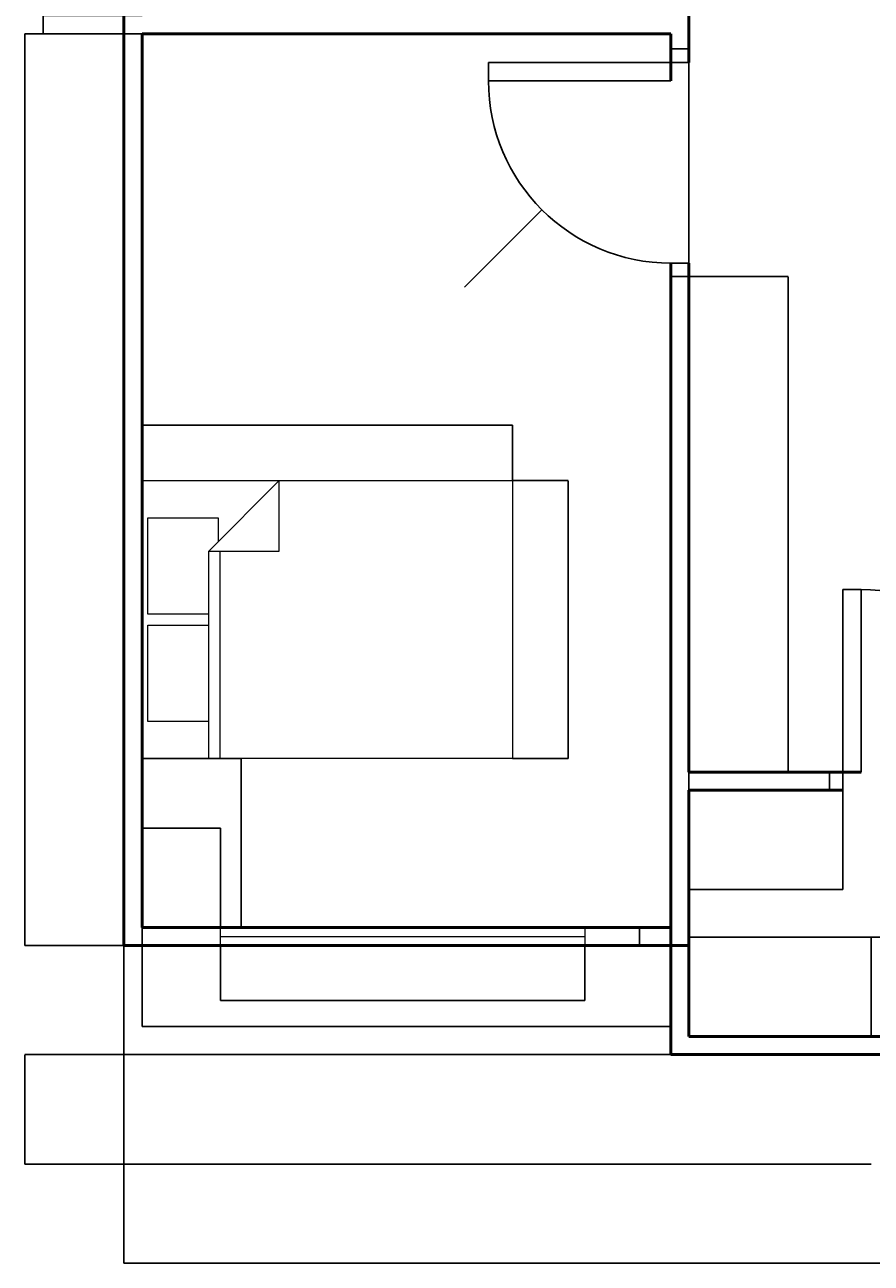
# Model space of a CAD drawing. Units: millimetres. Extents: x 1584 to 12772, y -932 to 10602.
# Tile 1 of 4: x 1584 to 6228, y -932 to 5860. Entities that reach past the tile are written whole.
import ezdxf

# ---------------------------------------------------------------- set-up
doc = ezdxf.new("R2010")
doc.units = ezdxf.units.MM
for name, color, linetype, lineweight in [('A-ANNO-DIMS', 2, 'Continuous', 18), ('A-DOOR', 3, 'Continuous', 25), ('A-FURN', 8, 'Continuous', 18), ('A-GLAZ', 4, 'Continuous', 18), ('A-WALL', 7, 'Continuous', 50)]:
    doc.layers.add(name, color=color, linetype=linetype, lineweight=lineweight)
doc.styles.get("Standard").update_dxf_attribs({"font": 'arial.ttf'})
doc.dimstyles.get("Standard").update_dxf_attribs({"dimtxt": 0.18, "dimasz": 0.18, "dimexe": 0.18, "dimexo": 0.0625, "dimgap": 0.09, "dimtad": 0, "dimtih": 1, "dimtoh": 1, "dimdec": 4, "dimzin": 0, "dimdsep": 46, "dimtxsty": 'Standard', "dimcen": 0.09, "dimadec": 0, "dimazin": 0, "dimtfac": 1, "dimtdec": 4, "dimtofl": 0, "dimtmove": 0, "dimatfit": 3, "dimfxl": 1, "dimtolj": 1, "dimtzin": 0, "dimarcsym": 0})

# ---------------------------------------------------------------- blocks, each defined once
blk = doc.blocks.new('Bed - Queen')
for p, q in [((0, -80.00003), (0, 0)), ((0, 0), (59.99999, 0)), ((59.99999, 0), (59.99999, -80.00003)), ((7.99999, -1.2), (28.79998, -1.2)), ((7.99999, -14.4), (7.99999, -1.2)), ((28.79998, -1.2), (28.79998, -14.4)), ((31.19999, -1.2), (51.99999, -1.2)), ((31.19999, -14.4), (31.19999, -1.2)), ((51.99999, -1.2), (51.99999, -16.4)), ((0, -14.4), (44.8, -14.4)), ((59.99999, -29.6), (44.8, -14.4)), ((44.8, -14.4), (44.8, -29.6)), ((44.8, -16.8), (0, -16.8)), ((51.99999, -16.4), (46.79936, -16.4)), ((44.8, -29.6), (59.99999, -29.6)), ((59.99999, -80.00003), (0, -80.00003))]:
    blk.add_line(p, q)
blk = doc.blocks.new('DOOR-SINGLE-1000')
for p, q in [((1000, 1174.2), (1000, 1248.4)), ((1000, 1248.4), (1100, 1248.4)), ((1100, 1248.4), (1100, 1174.2)), ((1000, 1174.2), (0, 1174.2)), ((0, 1174.2), (0, 1074.2)), ((1000, 1074.2), (1000, 1174.2)), ((1100, 1174.2), (1000, 1174.2)), ((0, 1074.2), (1000, 1074.2)), ((1000, 0), (1000, 74.2)), ((1000, 74.2), (1100, 74.2)), ((1100, 74.2), (1100, 0)), ((1100, 0), (1000, 0))]:
    blk.add_line(p, q)
blk.add_arc((1000, 1074.2), 1000, 180, 270)
blk = doc.blocks.new('DOOR-ENTRY-LEAF-1000')
for p, q in [((1100, 1100), (1000, 1100)), ((1000, 1100), (1000, 100)), ((1100, 100), (1100, 1100)), ((1000, 100), (1100, 100)), ((1100, 100), (1174.2, 100)), ((1100, 0), (1100, 100)), ((1174.2, 100), (1174.2, 0)), ((1174.2, 0), (1100, 0))]:
    blk.add_line(p, q)
blk.add_arc((1000, 100), 1000, 90, 180)
blk = doc.blocks.new('WIN-2000')
for p, q in [((0, 100), (2000, 100)), ((0, 0), (0, 100)), ((2000, 100), (2000, 0)), ((0, 50), (2000, 50)), ((2000, 0), (0, 0))]:
    blk.add_line(p, q)
blk = doc.blocks.new('*D14')
at = {"layer": 'A-ANNO-DIMS', "color": 0, "lineweight": -2, "transparency": 16777216}
for p, q in [((2657.2, 810.1), (2657.2, 510)), ((4657.2, 810.1), (4657.2, 510)), ((2657.4, 510.2), (3656, 510.2)), ((4657, 510.2), (3658.5, 510.2))]:
    blk.add_line(p, q, dxfattribs=at)
at = {"layer": 'A-ANNO-DIMS', "color": 0, "transparency": 16777216}
for points in [[(2657.4, 510.2), (2657.4, 510.2), (2657.2, 510.2)], [(4657, 510.2), (4657, 510.2), (4657.2, 510.2)]]:
    blk.add_solid(points, dxfattribs=at)
at = {"layer": 'Defpoints', "color": 0, "transparency": 16777216}
for p in [(2657.2, 810.2), (4657.2, 810.2), (4657.2, 510.2)]:
    blk.add_point(p, dxfattribs=at)
at = {"layer": 'A-ANNO-DIMS', "color": 0, "transparency": 16777216, "insert": (3657.2, 510.2), "char_height": 0.18, "attachment_point": 5}
blk.add_mtext('\\A1;WINDOW 2000 TYP.', dxfattribs=at)
blk = doc.blocks.new('*D15')
at = {"layer": 'A-ANNO-DIMS', "color": 0, "lineweight": -2, "transparency": 16777216}
for p, q in [((4657.3, 910.2), (4957.4, 910.2)), ((4957.2, 910), (4957.2, 860.4)), ((4957.2, 810.4), (4957.2, 860)), ((4657.3, 810.2), (4957.4, 810.2))]:
    blk.add_line(p, q, dxfattribs=at)
at = {"layer": 'A-ANNO-DIMS', "color": 0, "transparency": 16777216}
for points in [[(4957.2, 910), (4957.3, 910), (4957.2, 910.2)], [(4957.2, 810.4), (4957.3, 810.4), (4957.2, 810.2)]]:
    blk.add_solid(points, dxfattribs=at)
at = {"layer": 'Defpoints', "color": 0, "transparency": 16777216}
for p in [(4657.2, 910.2), (4957.2, 910.2), (4657.2, 810.2)]:
    blk.add_point(p, dxfattribs=at)
at = {"layer": 'A-ANNO-DIMS', "color": 0, "transparency": 16777216, "insert": (4957.2, 860.2), "char_height": 0.18, "attachment_point": 5}
blk.add_mtext('\\A1;100 TYP.', dxfattribs=at)
blk = doc.blocks.new('*D20')
at = {"layer": 'A-ANNO-DIMS', "color": 0, "lineweight": -2, "transparency": 16777216}
for p, q in [((2227.8, 3360.2), (2227.8, 3665.2)), ((2228, 3665), (3242.4, 3665)), ((4259.7, 3665), (3245.3, 3665)), ((4259.8, 3360.2), (4259.8, 3665.2))]:
    blk.add_line(p, q, dxfattribs=at)
at = {"layer": 'A-ANNO-DIMS', "color": 0, "transparency": 16777216}
for points in [[(2228, 3665), (2228, 3665), (2227.8, 3665)], [(4259.7, 3665), (4259.7, 3665), (4259.8, 3665)]]:
    blk.add_solid(points, dxfattribs=at)
at = {"layer": 'Defpoints', "color": 0, "transparency": 16777216}
for p in [(2227.8, 3665), (2227.8, 3360.2), (4259.8, 3360.2)]:
    blk.add_point(p, dxfattribs=at)
at = {"layer": 'A-ANNO-DIMS', "color": 0, "transparency": 16777216, "insert": (3243.8, 3665), "char_height": 0.18, "attachment_point": 5}
blk.add_mtext('\\A1;QUEEN BED 2032 TYP.', dxfattribs=at)
blk = doc.blocks.new('*D21')
at = {"layer": 'A-ANNO-DIMS', "color": 0, "lineweight": -2, "transparency": 16777216}
for p, q in [((4259.9, 3360.2), (4564.8, 3360.2)), ((4564.6, 3360), (4564.6, 2598.4)), ((4564.6, 1836.4), (4564.6, 2598)), ((4259.9, 1836.2), (4564.8, 1836.2))]:
    blk.add_line(p, q, dxfattribs=at)
at = {"layer": 'A-ANNO-DIMS', "color": 0, "transparency": 16777216}
for points in [[(4564.6, 3360), (4564.7, 3360), (4564.6, 3360.2)], [(4564.6, 1836.4), (4564.7, 1836.4), (4564.6, 1836.2)]]:
    blk.add_solid(points, dxfattribs=at)
at = {"layer": 'Defpoints', "color": 0, "transparency": 16777216}
for p in [(4259.8, 3360.2), (4564.6, 3360.2), (4259.8, 1836.2)]:
    blk.add_point(p, dxfattribs=at)
at = {"layer": 'A-ANNO-DIMS', "color": 0, "transparency": 16777216, "insert": (4564.6, 2598.2), "char_height": 0.18, "attachment_point": 5}
blk.add_mtext('\\A1;1524 TYP.', dxfattribs=at)
blk = doc.blocks.new('*D36')
at = {"layer": 'A-ANNO-DIMS', "color": 0, "lineweight": -2, "transparency": 16777216}
for p, q in [((2127.8, 810.1), (2127.8, -931.5)), ((12227.8, 810.1), (12227.8, -931.5)), ((2128, -931.3), (7177.4, -931.3)), ((12227.7, -931.3), (7178.3, -931.3))]:
    blk.add_line(p, q, dxfattribs=at)
at = {"layer": 'A-ANNO-DIMS', "color": 0, "transparency": 16777216}
for points in [[(2128, -931.3), (2128, -931.4), (2127.8, -931.3)], [(12227.7, -931.3), (12227.7, -931.4), (12227.8, -931.3)]]:
    blk.add_solid(points, dxfattribs=at)
at = {"layer": 'Defpoints', "color": 0, "transparency": 16777216}
for p in [(2127.8, 810.2), (12227.8, 810.2), (12227.8, -931.3)]:
    blk.add_point(p, dxfattribs=at)
at = {"layer": 'A-ANNO-DIMS', "color": 0, "transparency": 16777216, "insert": (7177.8, -931.3), "char_height": 0.18, "attachment_point": 5}
blk.add_mtext('\\A1;10100', dxfattribs=at)
blk = doc.blocks.new('*D38')
at = {"layer": 'A-ANNO-DIMS', "color": 0, "lineweight": -2, "transparency": 16777216}
for p, q in [((2227.8, 5810.2), (1584, 5810.2)), ((1584.1, 5810), (1584.1, 3310.4)), ((1584.1, 810.4), (1584.1, 3310)), ((2127.8, 810.2), (1584, 810.2))]:
    blk.add_line(p, q, dxfattribs=at)
at = {"layer": 'A-ANNO-DIMS', "color": 0, "transparency": 16777216}
for points in [[(1584.1, 5810), (1584.2, 5810), (1584.1, 5810.2)], [(1584.1, 810.4), (1584.2, 810.4), (1584.1, 810.2)]]:
    blk.add_solid(points, dxfattribs=at)
at = {"layer": 'Defpoints', "color": 0, "transparency": 16777216}
for p in [(1584.1, 5810.2), (2227.8, 5810.2), (2127.8, 810.2)]:
    blk.add_point(p, dxfattribs=at)
at = {"layer": 'A-ANNO-DIMS', "color": 0, "transparency": 16777216, "insert": (1584.1, 3310.2), "char_height": 0.18, "attachment_point": 5}
blk.add_mtext('\\A1;5000', dxfattribs=at)
blk = doc.blocks.new('*D40')
at = {"layer": 'A-ANNO-DIMS', "color": 0, "lineweight": -2, "transparency": 16777216}
for p, q in [((2227.8, 5910.2), (1684, 5910.2)), ((1684.1, 5910), (1684.1, 5860.4)), ((1684.1, 5810.4), (1684.1, 5860)), ((2227.8, 5810.2), (1684, 5810.2))]:
    blk.add_line(p, q, dxfattribs=at)
at = {"layer": 'A-ANNO-DIMS', "color": 0, "transparency": 16777216}
for points in [[(1684.1, 5910), (1684.2, 5910), (1684.1, 5910.2)], [(1684.1, 5810.4), (1684.2, 5810.4), (1684.1, 5810.2)]]:
    blk.add_solid(points, dxfattribs=at)
at = {"layer": 'Defpoints', "color": 0, "transparency": 16777216}
for p in [(1684.1, 5910.2), (2227.8, 5910.2), (2227.8, 5810.2)]:
    blk.add_point(p, dxfattribs=at)
at = {"layer": 'A-ANNO-DIMS', "color": 0, "transparency": 16777216, "insert": (1684.1, 5860.2), "char_height": 0.18, "attachment_point": 5}
blk.add_mtext('\\A1;100', dxfattribs=at)
blk = doc.blocks.new('*D43')
at = {"layer": 'A-ANNO-DIMS', "color": 0, "lineweight": -2, "transparency": 16777216}
for p, q in [((2227.83323, 910.118106), (2227.83323, 366.300606)), ((5127.83323, 910.118106), (5127.83323, 366.300606)), ((2228.01323, 366.480606), (3677.47323, 366.480606)), ((5127.65323, 366.480606), (3678.19323, 366.480606))]:
    blk.add_line(p, q, dxfattribs=at)
at = {"layer": 'A-ANNO-DIMS', "color": 0, "transparency": 16777216}
for points in [[(2228.01323, 366.510606), (2228.01323, 366.450606), (2227.83323, 366.480606)], [(5127.65323, 366.510606), (5127.65323, 366.450606), (5127.83323, 366.480606)]]:
    blk.add_solid(points, dxfattribs=at)
at = {"layer": 'Defpoints', "color": 0, "transparency": 16777216}
for p in [(2227.83323, 910.180606), (5127.83323, 910.180606), (2227.83323, 366.480606)]:
    blk.add_point(p, dxfattribs=at)
at = {"layer": 'A-ANNO-DIMS', "color": 0, "transparency": 16777216, "insert": (3677.83323, 366.480606), "char_height": 0.18, "attachment_point": 5}
blk.add_mtext('\\A1;2900', dxfattribs=at)
blk = doc.blocks.new('*D44')
at = {"layer": 'A-ANNO-DIMS', "color": 0, "lineweight": -2, "transparency": 16777216}
for p, q in [((5227.8, 312.4), (5227.8, 10454.1)), ((5228, 10453.9), (7177.5, 10453.9)), ((9127.7, 10453.9), (7178.2, 10453.9)), ((9127.8, 312.4), (9127.8, 10454.1))]:
    blk.add_line(p, q, dxfattribs=at)
at = {"layer": 'A-ANNO-DIMS', "color": 0, "transparency": 16777216}
for points in [[(5228, 10453.9), (5228, 10453.9), (5227.8, 10453.9)], [(9127.7, 10453.9), (9127.7, 10453.9), (9127.8, 10453.9)]]:
    blk.add_solid(points, dxfattribs=at)
at = {"layer": 'Defpoints', "color": 0, "transparency": 16777216}
for p in [(9127.8, 10453.9), (5227.8, 312.4), (9127.8, 312.4)]:
    blk.add_point(p, dxfattribs=at)
at = {"layer": 'A-ANNO-DIMS', "color": 0, "transparency": 16777216, "insert": (7177.8, 10453.9), "char_height": 0.18, "attachment_point": 5}
blk.add_mtext('\\A1;3900', dxfattribs=at)
blk = doc.blocks.new('*D47')
at = {"layer": 'A-ANNO-DIMS', "color": 0, "lineweight": -2, "transparency": 16777216}
for p, q in [((6227.83323, 312.424388), (6227.83323, 856.241888)), ((6228.01323, 856.061888), (7227.47323, 856.061888)), ((8227.65323, 856.061888), (7228.19323, 856.061888)), ((8227.83323, 312.424388), (8227.83323, 856.241888))]:
    blk.add_line(p, q, dxfattribs=at)
at = {"layer": 'A-ANNO-DIMS', "color": 0, "transparency": 16777216}
for points in [[(6228.01323, 856.091888), (6228.01323, 856.031888), (6227.83323, 856.061888)], [(8227.65323, 856.091888), (8227.65323, 856.031888), (8227.83323, 856.061888)]]:
    blk.add_solid(points, dxfattribs=at)
at = {"layer": 'Defpoints', "color": 0, "transparency": 16777216}
for p in [(8227.83323, 856.061888), (6227.83323, 312.361888), (8227.83323, 312.361888)]:
    blk.add_point(p, dxfattribs=at)
at = {"layer": 'A-ANNO-DIMS', "color": 0, "transparency": 16777216, "insert": (7227.83323, 856.061888), "char_height": 0.18, "attachment_point": 5}
blk.add_mtext('\\A1;2000', dxfattribs=at)
blk = doc.blocks.new('*D48')
at = {"layer": 'A-ANNO-DIMS', "color": 0, "lineweight": -2, "transparency": 16777216}
for p, q in [((5227.8, 312.4), (5227.8, 856.2)), ((5228, 856.1), (5727.5, 856.1)), ((6227.7, 856.1), (5728.2, 856.1)), ((6227.8, 312.4), (6227.8, 856.2))]:
    blk.add_line(p, q, dxfattribs=at)
at = {"layer": 'A-ANNO-DIMS', "color": 0, "transparency": 16777216}
for points in [[(5228, 856.1), (5228, 856), (5227.8, 856.1)], [(6227.7, 856.1), (6227.7, 856), (6227.8, 856.1)]]:
    blk.add_solid(points, dxfattribs=at)
at = {"layer": 'Defpoints', "color": 0, "transparency": 16777216}
for p in [(6227.8, 856.1), (5227.8, 312.4), (6227.8, 312.4)]:
    blk.add_point(p, dxfattribs=at)
at = {"layer": 'A-ANNO-DIMS', "color": 0, "transparency": 16777216, "insert": (5727.8, 856.1), "char_height": 0.18, "attachment_point": 5}
blk.add_mtext('\\A1;1000', dxfattribs=at)
blk = doc.blocks.new('*D49')
at = {"layer": 'A-ANNO-DIMS', "color": 0, "lineweight": -2, "transparency": 16777216}
for p, q in [((5127.8, 212.4), (1584, 212.4)), ((1584.1, 212.2), (1584.1, -87.5)), ((1584.1, -387.5), (1584.1, -87.8)), ((6227.8, -387.6), (1584, -387.6))]:
    blk.add_line(p, q, dxfattribs=at)
at = {"layer": 'A-ANNO-DIMS', "color": 0, "transparency": 16777216}
for points in [[(1584.1, 212.2), (1584.2, 212.2), (1584.1, 212.4)], [(1584.1, -387.5), (1584.2, -387.5), (1584.1, -387.6)]]:
    blk.add_solid(points, dxfattribs=at)
at = {"layer": 'Defpoints', "color": 0, "transparency": 16777216}
for p in [(5127.8, 212.4), (1584.1, -387.6), (6227.8, -387.6)]:
    blk.add_point(p, dxfattribs=at)
at = {"layer": 'A-ANNO-DIMS', "color": 0, "transparency": 16777216, "insert": (1584.1, -87.6), "char_height": 0.18, "attachment_point": 5}
blk.add_mtext('\\A1;600', dxfattribs=at)
blk = doc.blocks.new('*D50')
at = {"layer": 'A-ANNO-DIMS', "color": 0, "lineweight": -2, "transparency": 16777216}
for p, q in [((5227.8, 1662.3), (5227.8, 1118.5)), ((6072.8, 1662.3), (6072.8, 1118.5)), ((5228, 1118.7), (5650, 1118.7)), ((6072.6, 1118.7), (5650.6, 1118.7))]:
    blk.add_line(p, q, dxfattribs=at)
at = {"layer": 'A-ANNO-DIMS', "color": 0, "transparency": 16777216}
for points in [[(5228, 1118.7), (5228, 1118.6), (5227.8, 1118.7)], [(6072.6, 1118.7), (6072.6, 1118.6), (6072.8, 1118.7)]]:
    blk.add_solid(points, dxfattribs=at)
at = {"layer": 'Defpoints', "color": 0, "transparency": 16777216}
for p in [(5227.8, 1662.4), (6072.8, 1662.4), (5227.8, 1118.7)]:
    blk.add_point(p, dxfattribs=at)
at = {"layer": 'A-ANNO-DIMS', "color": 0, "transparency": 16777216, "insert": (5650.3, 1118.7), "char_height": 0.18, "attachment_point": 5}
blk.add_mtext('\\A1;845', dxfattribs=at)
blk = doc.blocks.new('*D54')
at = {"layer": 'A-ANNO-DIMS', "color": 0, "lineweight": -2, "transparency": 16777216}
for p, q in [((2227.8, 910.2), (2227.8, 1454.1)), ((2228, 1453.9), (2442.1, 1453.9)), ((2657, 1453.9), (2442.9, 1453.9)), ((2657.2, 910.2), (2657.2, 1454.1))]:
    blk.add_line(p, q, dxfattribs=at)
at = {"layer": 'A-ANNO-DIMS', "color": 0, "transparency": 16777216}
for points in [[(2228, 1453.9), (2228, 1453.9), (2227.8, 1453.9)], [(2657, 1453.9), (2657, 1453.9), (2657.2, 1453.9)]]:
    blk.add_solid(points, dxfattribs=at)
at = {"layer": 'Defpoints', "color": 0, "transparency": 16777216}
for p in [(2657.2, 1453.9), (2227.8, 910.2), (2657.2, 910.2)]:
    blk.add_point(p, dxfattribs=at)
at = {"layer": 'A-ANNO-DIMS', "color": 0, "transparency": 16777216, "insert": (2442.5, 1453.9), "char_height": 0.18, "attachment_point": 5}
blk.add_mtext('\\A1;429.4', dxfattribs=at)
blk = doc.blocks.new('*D57')
at = {"layer": 'A-ANNO-DIMS', "color": 0, "lineweight": -2, "transparency": 16777216}
for p, q in [((5227.9, 4478.9), (5771.7, 4478.9)), ((5771.5, 4478.7), (5771.5, 3120.8)), ((5771.5, 1762.5), (5771.5, 3120.5)), ((5227.9, 1762.4), (5771.7, 1762.4))]:
    blk.add_line(p, q, dxfattribs=at)
at = {"layer": 'A-ANNO-DIMS', "color": 0, "transparency": 16777216}
for points in [[(5771.5, 4478.7), (5771.6, 4478.7), (5771.5, 4478.9)], [(5771.5, 1762.5), (5771.6, 1762.5), (5771.5, 1762.4)]]:
    blk.add_solid(points, dxfattribs=at)
at = {"layer": 'Defpoints', "color": 0, "transparency": 16777216}
for p in [(5227.8, 4478.9), (5227.8, 1762.4), (5771.5, 1762.4)]:
    blk.add_point(p, dxfattribs=at)
at = {"layer": 'A-ANNO-DIMS', "color": 0, "transparency": 16777216, "insert": (5771.5, 3120.6), "char_height": 0.18, "attachment_point": 5}
blk.add_mtext('\\A1;2716.6', dxfattribs=at)
blk = doc.blocks.new('*D66')
at = {"layer": 'A-ANNO-DIMS', "color": 0, "lineweight": -2, "transparency": 16777216}
for p, q in [((2227.9, 1836.2), (2771.7, 1836.2)), ((2771.5, 1836), (2771.5, 1373.4)), ((2771.5, 910.4), (2771.5, 1373)), ((2227.9, 910.2), (2771.7, 910.2))]:
    blk.add_line(p, q, dxfattribs=at)
at = {"layer": 'A-ANNO-DIMS', "color": 0, "transparency": 16777216}
for points in [[(2771.5, 1836), (2771.6, 1836), (2771.5, 1836.2)], [(2771.5, 910.4), (2771.6, 910.4), (2771.5, 910.2)]]:
    blk.add_solid(points, dxfattribs=at)
at = {"layer": 'Defpoints', "color": 0, "transparency": 16777216}
for p in [(2227.8, 1836.2), (2227.8, 910.2), (2771.5, 910.2)]:
    blk.add_point(p, dxfattribs=at)
at = {"layer": 'A-ANNO-DIMS', "color": 0, "transparency": 16777216, "insert": (2771.5, 1373.2), "char_height": 0.18, "attachment_point": 5}
blk.add_mtext('\\A1;926', dxfattribs=at)
blk = doc.blocks.new('*D72')
at = {"layer": 'A-ANNO-DIMS', "color": 0, "lineweight": -2, "transparency": 16777216}
for p, q in [((5227.8, 4479), (5227.8, 10454.1)), ((5228, 10453.9), (6008.3, 10453.9)), ((6789.4, 10453.9), (6009.2, 10453.9)), ((6789.6, 4491.7), (6789.6, 10454.1))]:
    blk.add_line(p, q, dxfattribs=at)
at = {"layer": 'A-ANNO-DIMS', "color": 0, "transparency": 16777216}
for points in [[(5228, 10453.9), (5228, 10453.9), (5227.8, 10453.9)], [(6789.4, 10453.9), (6789.4, 10453.9), (6789.6, 10453.9)]]:
    blk.add_solid(points, dxfattribs=at)
at = {"layer": 'Defpoints', "color": 0, "transparency": 16777216}
for p in [(6789.6, 10453.9), (6789.6, 4491.7), (5227.8, 4478.9)]:
    blk.add_point(p, dxfattribs=at)
at = {"layer": 'A-ANNO-DIMS', "color": 0, "transparency": 16777216, "insert": (6008.7, 10453.9), "char_height": 0.18, "attachment_point": 5}
blk.add_mtext('\\A1;1561.8', dxfattribs=at)
blk = doc.blocks.new('*D80')
at = {"layer": 'A-ANNO-DIMS', "color": 0, "lineweight": -2, "transparency": 16777216}
for p, q in [((5127.7, 5553.1), (5127.9, 5553.1)), ((5127.8, 5553), (5127.8, 5553.2)), ((3996.5, 4421.7), (4420.6, 4845.9)), ((3996.3, 4421.7), (3996.5, 4421.7))]:
    blk.add_line(p, q, dxfattribs=at)
at = {"layer": 'A-ANNO-DIMS', "color": 0, "transparency": 16777216}
blk.add_solid([(4420.6, 4845.9), (4420.6, 4845.9), (4420.7, 4846)], dxfattribs=at)
at = {"layer": 'Defpoints', "color": 0, "transparency": 16777216}
for p in [(5127.8, 5553.1), (4420.7, 4846)]:
    blk.add_point(p, dxfattribs=at)
at = {"layer": 'A-ANNO-DIMS', "color": 0, "transparency": 16777216, "insert": (3995.6, 4421.7), "char_height": 0.18, "attachment_point": 5}
blk.add_mtext('\\A1;7X R1000', dxfattribs=at)

msp = doc.modelspace()

# ---------------------------------------------------------------- linework, layer by layer
at = {"layer": 'A-WALL'}
for p, q in [((2127.833, 9910.181), (2127.833, 810.181)), ((5227.833, 5910.181), (5227.833, 5810.181)), ((5127.833, 5810.181), (2227.833, 5810.181)), ((2227.833, 5810.181), (2227.833, 910.181)), ((5127.833, 5810.181), (5127.833, 5553.114)), ((5227.833, 5810.181), (5227.833, 5653.114)), ((5127.833, 4553.114), (5127.833, 910.181)), ((5227.833, 4553.114), (5227.833, 2410.181)), ((5227.833, 2310.181), (5227.833, 2410.181)), ((5227.833, 2310.181), (5227.833, 1762.362)), ((5227.833, 1762.362), (6172.821, 1762.362)), ((5227.833, 1662.362), (6072.821, 1662.362)), ((5227.833, 1662.362), (5227.833, 312.362)), ((5227.833, 1662.362), (5227.833, 910.181)), ((2227.833, 910.181), (5127.833, 910.181)), ((5127.833, 910.181), (5127.833, 212.362)), ((2127.833, 810.181), (5227.833, 810.181)), ((5127.833, 212.362), (5127.833, 312.362)), ((5227.833, 312.362), (9127.833, 312.362)), ((9127.833, 212.362), (5127.833, 212.362)), ((5227.833, 212.362), (9227.833, 212.362))]:
    msp.add_line(p, q, dxfattribs=at)

# ---------------------------------------------------------------- block references
at = {"layer": 'A-DOOR'}
msp.add_blockref('DOOR-SINGLE-1000', (4127.833, 4478.914), dxfattribs=at)
at = {"layer": 'A-DOOR', "extrusion": (0, 0, -1), "zscale": -1}
msp.add_blockref('DOOR-ENTRY-LEAF-1000', (-7172.82, 1662.362), dxfattribs=at)
at = {"layer": 'A-FURN', "xscale": 25.4, "yscale": 25.4, "zscale": 25.4, "rotation": 90}
msp.add_blockref('Bed - Queen', (2227.833, 1836.181), dxfattribs=at)
at = {"layer": 'A-GLAZ'}
msp.add_blockref('WIN-2000', (2657.227, 810.181), dxfattribs=at)

# ---------------------------------------------------------------- dimensions: what is measured, and where the dimension line sits
at = {"layer": 'A-ANNO-DIMS'}
for base, p1, p2, override, picture, middle in [((9127.833, 10453.881), (5227.833, 312.362), (9127.833, 312.362), {"dimdec": 0, "dimlfac": 1, "dimrnd": 0, "dimzin": 0, "dimdsep": 46, "dimlunit": 2}, '*D44', (7177.833, 10453.881)), ((6789.588, 10453.881), (5227.833, 4478.914), (6789.588, 4491.685), {"dimdec": 1, "dimlfac": 1, "dimrnd": 0, "dimzin": 0, "dimdsep": 46, "dimlunit": 2}, '*D72', (6008.711, 10453.881)), ((2657.226, 1453.881), (2227.833, 910.181), (2657.226, 910.181), {"dimdec": 1, "dimlfac": 1, "dimrnd": 0, "dimzin": 0, "dimdsep": 46, "dimlunit": 2}, '*D54', (2442.53, 1453.881)), ((6227.833, 856.062), (5227.833, 312.362), (6227.833, 312.362), {"dimdec": 0, "dimlfac": 1, "dimrnd": 0, "dimzin": 0, "dimdsep": 46, "dimlunit": 2}, '*D48', (5727.833, 856.062)), ((8227.833, 856.062), (6227.833, 312.362), (8227.833, 312.362), {"dimdec": 0, "dimlfac": 1, "dimrnd": 0, "dimzin": 0, "dimdsep": 46, "dimlunit": 2}, '*D47', (7227.833, 856.062)), ((12227.833, -931.338), (2127.833, 810.181), (12227.833, 810.181), {"dimdec": 0, "dimlfac": 1, "dimrnd": 0, "dimzin": 0, "dimdsep": 46, "dimlunit": 2}, '*D36', (7177.833, -931.338))]:
    dim = msp.add_linear_dim(base=base, p1=p1, p2=p2, dimstyle='Standard', override=override, dxfattribs=at)
    dim.commit()
    dim.dimension.update_dxf_attribs({"geometry": picture, "text_midpoint": middle})
for base, p1, p2, angle, override, picture, middle in [((1684.133, 5910.181), (2227.833, 5810.181), (2227.833, 5910.181), 90, {"dimdec": 0, "dimlfac": 1, "dimrnd": 0, "dimzin": 0, "dimdsep": 46, "dimlunit": 2}, '*D40', (1684.133, 5860.181)), ((1584.133, 5810.181), (2127.833, 810.181), (2227.833, 5810.181), 90, {"dimdec": 0, "dimlfac": 1, "dimrnd": 0, "dimzin": 0, "dimdsep": 46, "dimlunit": 2}, '*D38', (1584.133, 3310.181)), ((5771.533, 1762.362), (5227.833, 4478.914), (5227.833, 1762.362), 270, {"dimdec": 1, "dimlfac": 1, "dimrnd": 0, "dimzin": 0, "dimdsep": 46, "dimlunit": 2}, '*D57', (5771.533, 3120.638)), ((2771.533, 910.181), (2227.833, 1836.181), (2227.833, 910.181), 270, {"dimdec": 0, "dimlfac": 1, "dimrnd": 0, "dimzin": 0, "dimdsep": 46, "dimlunit": 2}, '*D66', (2771.533, 1373.181)), ((5227.833, 1118.662), (6072.821, 1662.362), (5227.833, 1662.362), 180, {"dimdec": 0, "dimlfac": 1, "dimrnd": 0, "dimzin": 0, "dimdsep": 46, "dimlunit": 2}, '*D50', (5650.327, 1118.662)), ((2227.833, 366.481), (5127.833, 910.181), (2227.833, 910.181), 180, {"dimdec": 0, "dimlfac": 1, "dimrnd": 0, "dimzin": 0, "dimdsep": 46, "dimlunit": 2}, '*D43', (3677.833, 366.481)), ((1584.133, -387.638), (5127.833, 212.362), (6227.833, -387.638), 90, {"dimdec": 0, "dimlfac": 1, "dimrnd": 0, "dimzin": 0, "dimdsep": 46, "dimlunit": 2}, '*D49', (1584.133, -87.638))]:
    dim = msp.add_linear_dim(base=base, p1=p1, p2=p2, angle=angle, dimstyle='Standard', override=override, dxfattribs=at)
    dim.commit()
    dim.dimension.update_dxf_attribs({"geometry": picture, "text_midpoint": middle})
dim = msp.add_radius_dim(center=(5127.833, 5553.114), mpoint=(4420.726, 4846.007), text='7X <>', dimstyle='Standard', override={"dimdec": 0, "dimlfac": 1, "dimrnd": 0, "dimzin": 0, "dimdsep": 46, "dimlunit": 2}, dxfattribs=at)
dim.commit()
dim.dimension.update_dxf_attribs({"geometry": '*D80', "text_midpoint": (3995.645, 4421.743), "dimtype": 164})
for base, p1, p2, angle, text, picture, middle in [((2227.833, 3664.981), (4259.834, 3360.181), (2227.833, 3360.181), 180, 'QUEEN BED <> TYP.', '*D20', (3243.834, 3664.981)), ((4564.634, 3360.181), (4259.834, 1836.181), (4259.834, 3360.181), 90, '<> TYP.', '*D21', (4564.634, 2598.181)), ((4957.226, 910.181), (4657.226, 810.181), (4657.226, 910.181), 90, '<> TYP.', '*D15', (4957.226, 860.181))]:
    dim = msp.add_linear_dim(base=base, p1=p1, p2=p2, angle=angle, text=text, dimstyle='Standard', override={"dimdec": 0, "dimlfac": 1, "dimrnd": 0, "dimzin": 0, "dimdsep": 46, "dimlunit": 2}, dxfattribs=at)
    dim.commit()
    dim.dimension.update_dxf_attribs({"geometry": picture, "text_midpoint": middle})
dim = msp.add_linear_dim(base=(4657.226, 510.181), p1=(2657.226, 810.181), p2=(4657.226, 810.181), text='WINDOW <> TYP.', dimstyle='Standard', override={"dimdec": 0, "dimlfac": 1, "dimrnd": 0, "dimzin": 0, "dimdsep": 46, "dimlunit": 2}, dxfattribs=at)
dim.commit()
dim.dimension.update_dxf_attribs({"geometry": '*D14', "text_midpoint": (3657.226, 510.181)})

doc.saveas('drawing.dxf')
